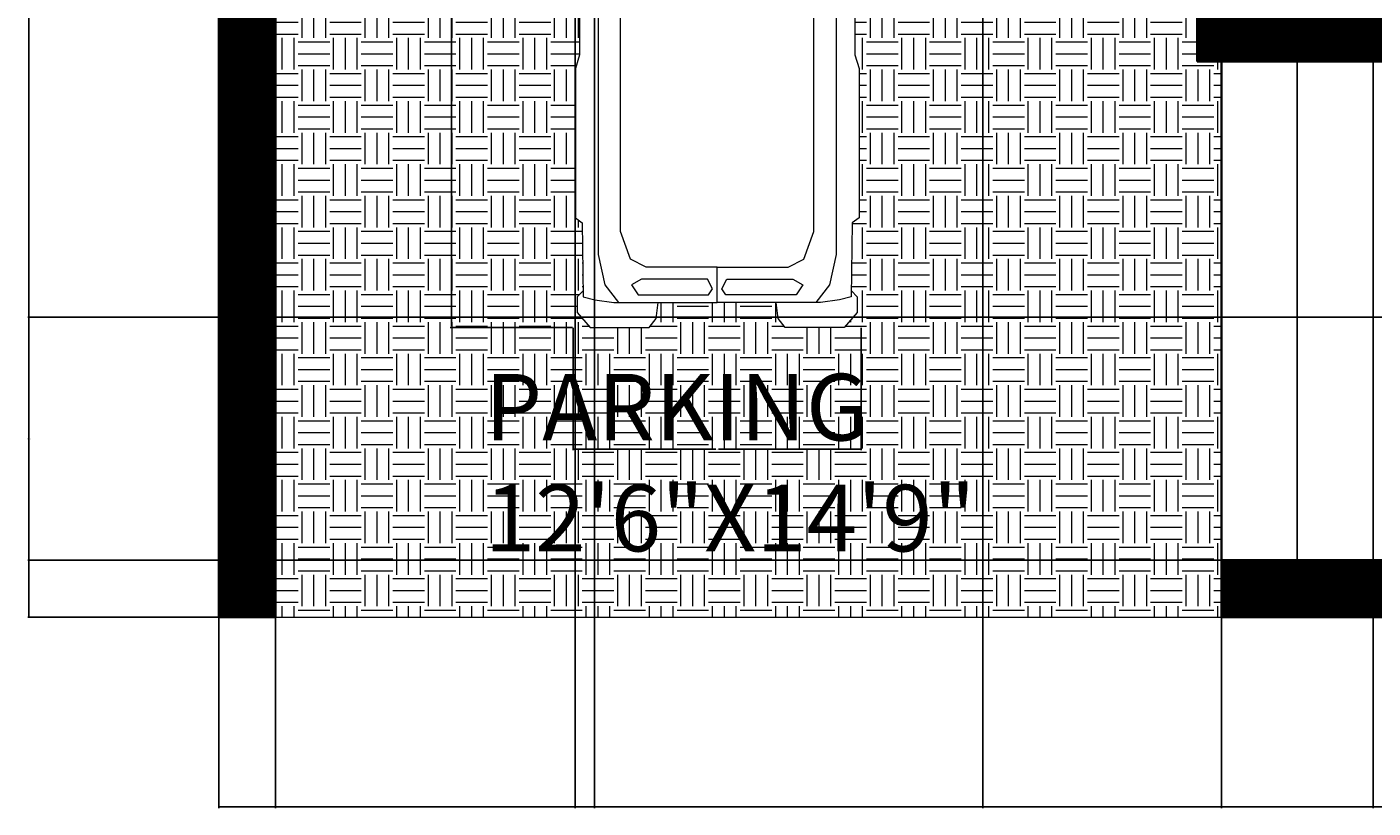
# Model space of a CAD drawing. Units: inches. Extents: x 205 to 1667, y -23 to 828.
# Tile 1 of 10: x 432 to 645, y -23 to 101. Entities that reach past the tile are written whole.
import ezdxf

# ---------------------------------------------------------------- set-up
doc = ezdxf.new("R2010")
doc.units = ezdxf.units.IN
doc.header["$MEASUREMENT"] = 0
for name, color, linetype, lineweight in [('A-ANNO-DIMS', 2, 'Continuous', 18), ('A-AREA-IDEN', 7, 'Continuous', 25), ('A-FLOR-PKNG', 8, 'Continuous', 18), ('A-FLOR-STRS', 7, 'Continuous', 25), ('A-WALL', 7, 'Continuous', 35)]:
    doc.layers.add(name, color=color, linetype=linetype, lineweight=lineweight)
doc.layers.add('A-FLOR-PATT', color=9, linetype='Continuous', lineweight=9, true_color=0xc7c8ca)
doc.styles.get("Standard").update_dxf_attribs({"font": 'arial.ttf'})
doc.dimstyles.get("Standard").update_dxf_attribs({"dimtxt": 0.18, "dimasz": 0.18, "dimexe": 0.18, "dimexo": 0.0625, "dimgap": 0.09, "dimtad": 0, "dimtih": 1, "dimtoh": 1, "dimdec": 4, "dimzin": 0, "dimdsep": 46, "dimtxsty": 'Standard', "dimcen": 0.09, "dimadec": 0, "dimazin": 0, "dimtfac": 1, "dimtdec": 4, "dimtofl": 0, "dimtmove": 0, "dimatfit": 3, "dimfxl": 1, "dimtolj": 1, "dimtzin": 0, "dimarcsym": 0})

# ---------------------------------------------------------------- blocks, each defined once
blk = doc.blocks.new('A$C3BDD66A0')
for p, q in [((-1.6934, 0.7345), (-1.7501, 0.6077)), ((-1.5608, 0.7448), (-1.6934, 0.7345)), ((-1.5055, 0.6573), (-1.5608, 0.7448)), ((-1.383, 0.6896), (-1.3262, 0.7247)), ((-1.3262, 0.7247), (-0.6328, 0.7247)), ((-0.6328, 0.7247), (-0.5818, 0.7108)), ((-0.5818, 0.7108), (1.0338, 0.7108)), ((0.0405, 0.522), (-0.2453, 0.7108)), ((1.0338, 0.7108), (1.1052, 0.7328)), ((1.1052, 0.7328), (1.8759, 0.7328)), ((1.8759, 0.7328), (1.9021, 0.6971)), ((1.9021, 0.6971), (2.2838, 0.6931)), ((2.2533, 0.6934), (2.2838, 0.7237)), ((2.2838, 0.7237), (2.3654, 0.7238)), ((2.3654, 0.7238), (2.4427, 0.6569)), ((-1.6379, 0.6224), (-1.383, 0.6896)), ((2.2838, 0.6931), (2.2999, 0.6319)), ((2.2999, 0.6319), (2.3146, 0.5344)), ((2.4427, 0.6569), (2.4427, 0.3509)), ((-1.7501, 0.6077), (-1.7501, 0)), ((-1.6275, 0.3471), (-1.6379, 0.6224)), ((-0.363, 0.4561), (-0.2962, 0.6237)), ((-0.363, 0.4561), (-0.2962, 0.6237)), ((-0.2962, 0.6237), (-0.2204, 0.599)), ((-0.2962, 0.6237), (-0.2204, 0.599)), ((-0.2204, 0.599), (0.0303, 0.4462)), ((-0.2204, 0.599), (0.0303, 0.4462)), ((-0.0842, 0.6044), (0.6056, 0.6044)), ((0.6056, 0.6044), (0.6056, 0.499)), ((0.6523, 0.6144), (2.0654, 0.6144)), ((0.6523, 0.499), (0.6523, 0.6144)), ((2.0654, 0.6144), (2.2228, 0.5809)), ((2.2228, 0.5809), (2.3146, 0.5096)), ((-1.6296, 0.403), (-1.0973, 0.5311)), ((-1.0973, 0.5311), (-0.4592, 0.5317)), ((-0.4592, 0.5317), (-0.4952, 0)), ((0.1935, 0.499), (0.0405, 0.522)), ((1.9475, 0.499), (0.1935, 0.499)), ((2.0903, 0.4482), (1.9475, 0.499)), ((2.3146, 0.5344), (2.3146, 0)), ((-0.4282, 0), (-0.363, 0.4561)), ((-0.4282, 0), (-0.363, 0.4561)), ((0.0303, 0.4462), (0.0654, 0.3691)), ((0.0303, 0.4462), (0.0654, 0.3691)), ((2.1315, 0.3666), (2.0903, 0.4482)), ((2.1927, 0.3914), (2.2229, 0.4425)), ((2.2229, 0.4425), (2.2739, 0.4076)), ((0.0654, 0.3691), (0, 0.1752)), ((0.0654, 0.3691), (0, 0.1752)), ((2.1315, 0), (2.1315, 0.3666)), ((2.1927, 0.0506), (2.1927, 0.3914)), ((2.2739, 0.4076), (2.2742, 0.0448)), ((2.4427, 0.3509), (2.3964, 0.3159)), ((-1.6519, 0), (-1.6275, 0.3471)), ((2.3964, 0.3159), (2.3146, 0.3056)), ((0, 0.1752), (0, 0)), ((0, 0.1752), (0, 0)), ((-1.7501, -0.6077), (-1.7501, 0)), ((-1.6519, 0), (-1.6275, -0.3471)), ((-1.4334, 0), (-0.4906, 0.0678)), ((-1.4334, 0), (-0.4906, -0.0678)), ((-0.4592, -0.5317), (-0.4952, 0)), ((-0.4282, 0), (-0.363, -0.4561)), ((-0.4282, 0), (-0.363, -0.4561)), ((0, -0.1752), (0, 0)), ((0, -0.1752), (0, 0)), ((2.1315, 0), (2.1315, -0.3666)), ((2.3146, 0), (2.1315, 0)), ((2.2437, 0.0244), (2.1927, 0.0506)), ((2.2742, 0.0448), (2.2437, 0.0244)), ((2.3146, -0.5344), (2.3146, 0)), ((2.2437, -0.0244), (2.1927, -0.0506)), ((2.1927, -0.0506), (2.1927, -0.3914)), ((2.2742, -0.0448), (2.2437, -0.0244)), ((2.2739, -0.4076), (2.2742, -0.0448)), ((0.0654, -0.3691), (0, -0.1752)), ((0.0654, -0.3691), (0, -0.1752)), ((-1.6275, -0.3471), (-1.6379, -0.6224)), ((2.3964, -0.3159), (2.3146, -0.3056)), ((2.4427, -0.3509), (2.3964, -0.3159)), ((-1.6296, -0.403), (-1.0973, -0.5311)), ((0.0303, -0.4462), (0.0654, -0.3691)), ((0.0303, -0.4462), (0.0654, -0.3691)), ((2.1315, -0.3666), (2.0903, -0.4482)), ((2.1927, -0.3914), (2.2229, -0.4425)), ((2.2229, -0.4425), (2.2739, -0.4076)), ((2.4427, -0.6569), (2.4427, -0.3509)), ((-0.363, -0.4561), (-0.2962, -0.6237)), ((-0.363, -0.4561), (-0.2962, -0.6237)), ((-0.2204, -0.599), (0.0303, -0.4462)), ((-0.2204, -0.599), (0.0303, -0.4462)), ((2.0903, -0.4482), (1.9475, -0.499)), ((-1.0973, -0.5311), (-0.4592, -0.5317)), ((0.0405, -0.522), (-0.2453, -0.7108)), ((0.1935, -0.499), (0.0405, -0.522)), ((1.9475, -0.499), (0.1935, -0.499)), ((0.6056, -0.6044), (0.6056, -0.499)), ((0.6523, -0.499), (0.6523, -0.6144)), ((2.2228, -0.5809), (2.3146, -0.5096)), ((2.2999, -0.6319), (2.3146, -0.5344)), ((-1.6934, -0.7345), (-1.7501, -0.6077)), ((-1.6379, -0.6224), (-1.383, -0.6896)), ((-0.2962, -0.6237), (-0.2204, -0.599)), ((-0.2962, -0.6237), (-0.2204, -0.599)), ((-0.0842, -0.6044), (0.6056, -0.6044)), ((0.6523, -0.6144), (2.0654, -0.6144)), ((2.0654, -0.6144), (2.2228, -0.5809)), ((-1.5055, -0.6573), (-1.5608, -0.7448)), ((-1.383, -0.6896), (-1.3262, -0.7247)), ((1.9021, -0.6971), (2.2838, -0.6931)), ((2.2533, -0.6934), (2.2838, -0.7237)), ((2.2838, -0.6931), (2.2999, -0.6319)), ((2.3654, -0.7238), (2.4427, -0.6569)), ((-1.5608, -0.7448), (-1.6934, -0.7345)), ((-1.3262, -0.7247), (-0.6328, -0.7247)), ((-0.6328, -0.7247), (-0.5818, -0.7108)), ((-0.5818, -0.7108), (1.0338, -0.7108)), ((1.0338, -0.7108), (1.1052, -0.7328)), ((1.1052, -0.7328), (1.8759, -0.7328)), ((1.8759, -0.7328), (1.9021, -0.6971)), ((2.2838, -0.7237), (2.3654, -0.7238))]:
    blk.add_line(p, q)
blk = doc.blocks.new('*D40')
at = {"layer": 'A-ANNO-DIMS', "color": 0, "lineweight": -2, "transparency": 16777216}
for p, q in [((518.48, 182.02), (499.09, 182.02)), ((499.27, 181.84), (499.27, 117.96)), ((499.27, 53.72), (499.27, 117.59)), ((518.48, 53.54), (499.09, 53.54))]:
    blk.add_line(p, q, dxfattribs=at)
at = {"layer": 'A-ANNO-DIMS', "color": 0, "transparency": 16777216}
for points in [[(499.24, 181.84), (499.3, 181.84), (499.27, 182.02)], [(499.24, 53.72), (499.3, 53.72), (499.27, 53.54)]]:
    blk.add_solid(points, dxfattribs=at)
at = {"layer": 'Defpoints', "color": 0, "transparency": 16777216}
for p in [(518.54, 182.02), (499.27, 53.54), (518.54, 53.54)]:
    blk.add_point(p, dxfattribs=at)
at = {"layer": 'A-ANNO-DIMS', "color": 0, "transparency": 16777216, "insert": (499.27, 117.78), "char_height": 0.18, "attachment_point": 5}
blk.add_mtext('\\A1;CAR 128', dxfattribs=at)
blk = doc.blocks.new('*D41')
at = {"layer": 'A-ANNO-DIMS', "color": 0, "lineweight": -2, "transparency": 16777216}
for p, q in [((518.54, 53.48), (518.54, 34.09)), ((564.19, 53.48), (564.19, 34.09)), ((518.72, 34.27), (541.14, 34.27)), ((564.01, 34.27), (541.59, 34.27))]:
    blk.add_line(p, q, dxfattribs=at)
at = {"layer": 'A-ANNO-DIMS', "color": 0, "transparency": 16777216}
for points in [[(518.72, 34.3), (518.72, 34.24), (518.54, 34.27)], [(564.01, 34.3), (564.01, 34.24), (564.19, 34.27)]]:
    blk.add_solid(points, dxfattribs=at)
at = {"layer": 'Defpoints', "color": 0, "transparency": 16777216}
for p in [(518.54, 53.54), (564.19, 53.54), (564.19, 34.27)]:
    blk.add_point(p, dxfattribs=at)
at = {"layer": 'A-ANNO-DIMS', "color": 0, "transparency": 16777216, "insert": (541.37, 34.27), "char_height": 0.18, "attachment_point": 5}
blk.add_mtext('\\A1;46', dxfattribs=at)
blk = doc.blocks.new('*D42')
at = {"layer": 'A-ANNO-DIMS', "color": 0, "lineweight": -2, "transparency": 16777216}
for p, q in [((462.43, 7.59), (462.43, -22.59)), ((774.43, 7.59), (774.43, -22.59)), ((462.61, -22.41), (618.14, -22.41)), ((774.25, -22.41), (618.72, -22.41))]:
    blk.add_line(p, q, dxfattribs=at)
at = {"layer": 'A-ANNO-DIMS', "color": 0, "transparency": 16777216}
for points in [[(462.61, -22.38), (462.61, -22.44), (462.43, -22.41)], [(774.25, -22.38), (774.25, -22.44), (774.43, -22.41)]]:
    blk.add_solid(points, dxfattribs=at)
at = {"layer": 'Defpoints', "color": 0, "transparency": 16777216}
for p in [(462.43, 7.65), (774.43, 7.65), (774.43, -22.41)]:
    blk.add_point(p, dxfattribs=at)
at = {"layer": 'A-ANNO-DIMS', "color": 0, "transparency": 16777216, "insert": (618.43, -22.41), "char_height": 0.18, "attachment_point": 5}
blk.add_mtext('\\A1;312', dxfattribs=at)
blk = doc.blocks.new('*D43')
at = {"layer": 'A-ANNO-DIMS', "color": 0, "lineweight": -2, "transparency": 16777216}
for p, q in [((462.37, 607.65), (432.19, 607.65)), ((432.37, 607.47), (432.37, 307.83)), ((432.37, 7.83), (432.37, 307.47)), ((462.37, 7.65), (432.19, 7.65))]:
    blk.add_line(p, q, dxfattribs=at)
at = {"layer": 'A-ANNO-DIMS', "color": 0, "transparency": 16777216}
for points in [[(432.34, 607.47), (432.4, 607.47), (432.37, 607.65)], [(432.34, 7.83), (432.4, 7.83), (432.37, 7.65)]]:
    blk.add_solid(points, dxfattribs=at)
at = {"layer": 'Defpoints', "color": 0, "transparency": 16777216}
for p in [(432.37, 607.65), (462.43, 607.65), (462.43, 7.65)]:
    blk.add_point(p, dxfattribs=at)
at = {"layer": 'A-ANNO-DIMS', "color": 0, "transparency": 16777216, "insert": (432.37, 307.65), "char_height": 0.18, "attachment_point": 5}
blk.add_mtext('\\A1;600', dxfattribs=at)
blk = doc.blocks.new('*D44')
at = {"layer": 'A-ANNO-DIMS', "color": 0, "lineweight": -2, "transparency": 16777216}
for p, q in [((462.43, 7.59), (462.43, -22.59)), ((621.22, 7.59), (621.22, -22.59)), ((462.61, -22.41), (541.44, -22.41)), ((621.04, -22.41), (542.21, -22.41))]:
    blk.add_line(p, q, dxfattribs=at)
at = {"layer": 'A-ANNO-DIMS', "color": 0, "transparency": 16777216}
for points in [[(462.61, -22.38), (462.61, -22.44), (462.43, -22.41)], [(621.04, -22.38), (621.04, -22.44), (621.22, -22.41)]]:
    blk.add_solid(points, dxfattribs=at)
at = {"layer": 'Defpoints', "color": 0, "transparency": 16777216}
for p in [(462.43, 7.65), (621.22, 7.65), (621.22, -22.41)]:
    blk.add_point(p, dxfattribs=at)
at = {"layer": 'A-ANNO-DIMS', "color": 0, "transparency": 16777216, "insert": (541.83, -22.41), "char_height": 0.18, "attachment_point": 5}
blk.add_mtext('\\A1;158.8', dxfattribs=at)
blk = doc.blocks.new('*D52')
at = {"layer": 'A-ANNO-DIMS', "color": 0, "lineweight": -2, "transparency": 16777216}
for p, q in [((471.43, 204.87), (471.43, -22.59)), ((521.94, 204.87), (521.94, -22.59)), ((471.61, -22.41), (496.36, -22.41)), ((521.76, -22.41), (497.01, -22.41))]:
    blk.add_line(p, q, dxfattribs=at)
at = {"layer": 'A-ANNO-DIMS', "color": 0, "transparency": 16777216}
for points in [[(471.61, -22.38), (471.61, -22.44), (471.43, -22.41)], [(521.76, -22.38), (521.76, -22.44), (521.94, -22.41)]]:
    blk.add_solid(points, dxfattribs=at)
at = {"layer": 'Defpoints', "color": 0, "transparency": 16777216}
for p in [(471.43, 204.93), (521.94, 204.93), (521.94, -22.41)]:
    blk.add_point(p, dxfattribs=at)
at = {"layer": 'A-ANNO-DIMS', "color": 0, "transparency": 16777216, "insert": (496.68, -22.41), "char_height": 0.18, "attachment_point": 5}
blk.add_mtext('\\A1;50.5', dxfattribs=at)
blk = doc.blocks.new('*D55')
at = {"layer": 'A-ANNO-DIMS', "color": 0, "lineweight": -2, "transparency": 16777216}
for p, q in [((621.22, 16.71), (621.22, 637.89)), ((621.4, 637.71), (627.01, 637.71)), ((633.04, 637.71), (627.43, 637.71)), ((633.22, 16.71), (633.22, 637.89))]:
    blk.add_line(p, q, dxfattribs=at)
at = {"layer": 'A-ANNO-DIMS', "color": 0, "transparency": 16777216}
for points in [[(621.4, 637.74), (621.4, 637.68), (621.22, 637.71)], [(633.04, 637.74), (633.04, 637.68), (633.22, 637.71)]]:
    blk.add_solid(points, dxfattribs=at)
at = {"layer": 'Defpoints', "color": 0, "transparency": 16777216}
for p in [(633.22, 637.71), (621.22, 16.65), (633.22, 16.65)]:
    blk.add_point(p, dxfattribs=at)
at = {"layer": 'A-ANNO-DIMS', "color": 0, "transparency": 16777216, "insert": (627.22, 637.71), "char_height": 0.18, "attachment_point": 5}
blk.add_mtext('\\A1;12', dxfattribs=at)
blk = doc.blocks.new('*D56')
at = {"layer": 'A-ANNO-DIMS', "color": 0, "lineweight": -2, "transparency": 16777216}
for p, q in [((621.16, 55.14), (432.19, 55.14)), ((432.37, 54.96), (432.37, 36.08)), ((432.37, 16.83), (432.37, 35.72)), ((621.16, 16.65), (432.19, 16.65))]:
    blk.add_line(p, q, dxfattribs=at)
at = {"layer": 'A-ANNO-DIMS', "color": 0, "transparency": 16777216}
for points in [[(432.34, 54.96), (432.4, 54.96), (432.37, 55.14)], [(432.34, 16.83), (432.4, 16.83), (432.37, 16.65)]]:
    blk.add_solid(points, dxfattribs=at)
at = {"layer": 'Defpoints', "color": 0, "transparency": 16777216}
for p in [(432.37, 55.14), (621.22, 55.14), (621.22, 16.65)]:
    blk.add_point(p, dxfattribs=at)
at = {"layer": 'A-ANNO-DIMS', "color": 0, "transparency": 16777216, "insert": (432.37, 35.9), "char_height": 0.18, "attachment_point": 5}
blk.add_mtext('\\A1;38.49', dxfattribs=at)
blk = doc.blocks.new('*D57')
at = {"layer": 'A-ANNO-DIMS', "color": 0, "lineweight": -2, "transparency": 16777216}
for p, q in [((621.22, 95.58), (621.22, -22.59)), ((645.22, 95.58), (645.22, -22.59)), ((621.4, -22.41), (633, -22.41)), ((645.04, -22.41), (633.44, -22.41))]:
    blk.add_line(p, q, dxfattribs=at)
at = {"layer": 'A-ANNO-DIMS', "color": 0, "transparency": 16777216}
for points in [[(621.4, -22.38), (621.4, -22.44), (621.22, -22.41)], [(645.04, -22.38), (645.04, -22.44), (645.22, -22.41)]]:
    blk.add_solid(points, dxfattribs=at)
at = {"layer": 'Defpoints', "color": 0, "transparency": 16777216}
for p in [(621.22, 95.64), (645.22, 95.64), (645.22, -22.41)]:
    blk.add_point(p, dxfattribs=at)
at = {"layer": 'A-ANNO-DIMS', "color": 0, "transparency": 16777216, "insert": (633.22, -22.41), "char_height": 0.18, "attachment_point": 5}
blk.add_mtext('\\A1;24', dxfattribs=at)
blk = doc.blocks.new('*D64')
at = {"layer": 'A-ANNO-DIMS', "color": 0, "lineweight": -2, "transparency": 16777216}
for p, q in [((471.43, 454.59), (471.43, -22.59)), ((583.44, 454.59), (583.44, -22.59)), ((471.61, -22.41), (527.16, -22.41)), ((583.26, -22.41), (527.71, -22.41))]:
    blk.add_line(p, q, dxfattribs=at)
at = {"layer": 'A-ANNO-DIMS', "color": 0, "transparency": 16777216}
for points in [[(471.61, -22.38), (471.61, -22.44), (471.43, -22.41)], [(583.26, -22.38), (583.26, -22.44), (583.44, -22.41)]]:
    blk.add_solid(points, dxfattribs=at)
at = {"layer": 'Defpoints', "color": 0, "transparency": 16777216}
for p in [(471.43, 454.65), (583.44, 454.65), (583.44, -22.41)]:
    blk.add_point(p, dxfattribs=at)
at = {"layer": 'A-ANNO-DIMS', "color": 0, "transparency": 16777216, "insert": (527.44, -22.41), "char_height": 0.18, "attachment_point": 5}
blk.add_mtext('\\A1;112', dxfattribs=at)
blk = doc.blocks.new('*D82')
at = {"layer": 'A-ANNO-DIMS', "color": 0, "lineweight": -2, "transparency": 16777216}
for p, q in [((471.43, 204.87), (471.43, -22.59)), ((518.86, 180.22), (518.86, -22.59)), ((471.61, -22.41), (494.75, -22.41)), ((518.68, -22.41), (495.54, -22.41))]:
    blk.add_line(p, q, dxfattribs=at)
at = {"layer": 'A-ANNO-DIMS', "color": 0, "transparency": 16777216}
for points in [[(471.61, -22.38), (471.61, -22.44), (471.43, -22.41)], [(518.68, -22.38), (518.68, -22.44), (518.86, -22.41)]]:
    blk.add_solid(points, dxfattribs=at)
at = {"layer": 'Defpoints', "color": 0, "transparency": 16777216}
for p in [(471.43, 204.93), (518.86, 180.28), (518.86, -22.41)]:
    blk.add_point(p, dxfattribs=at)
at = {"layer": 'A-ANNO-DIMS', "color": 0, "transparency": 16777216, "insert": (495.14, -22.41), "char_height": 0.18, "attachment_point": 5}
blk.add_mtext('\\A1;47.43', dxfattribs=at)
blk = doc.blocks.new('*D84')
at = {"layer": 'A-ANNO-DIMS', "color": 0, "lineweight": -2, "transparency": 16777216}
for p, q in [((471.37, 204.93), (432.19, 204.93)), ((432.37, 204.75), (432.37, 106.47)), ((432.37, 7.83), (432.37, 106.11)), ((471.37, 7.65), (432.19, 7.65))]:
    blk.add_line(p, q, dxfattribs=at)
at = {"layer": 'A-ANNO-DIMS', "color": 0, "transparency": 16777216}
for points in [[(432.34, 204.75), (432.4, 204.75), (432.37, 204.93)], [(432.34, 7.83), (432.4, 7.83), (432.37, 7.65)]]:
    blk.add_solid(points, dxfattribs=at)
at = {"layer": 'Defpoints', "color": 0, "transparency": 16777216}
for p in [(432.37, 204.93), (471.43, 204.93), (471.43, 7.65)]:
    blk.add_point(p, dxfattribs=at)
at = {"layer": 'A-ANNO-DIMS', "color": 0, "transparency": 16777216, "insert": (432.37, 106.29), "char_height": 0.18, "attachment_point": 5}
blk.add_mtext('\\A1;197.3', dxfattribs=at)

msp = doc.modelspace()

# ---------------------------------------------------------------- hatches: boundary and pattern name
at = {"layer": 'A-FLOR-PATT'}
h = msp.add_hatch(dxfattribs=at)
h.set_pattern_fill('ANSI31', color=256)
h.paths.add_polyline_path([(774.4305, 607.6511), (720.5338, 607.6511), (720.5338, 598.6511), (727.9933, 598.6511), (746.8614, 598.6511), (765.4305, 598.6511), (765.4305, 454.6511), (759.5298, 454.6511), (759.5298, 448.9635), (765.4305, 448.9635), (765.4305, 428.0602), (774.4305, 428.0602)])
h.paths.add_polyline_path([(765.4305, 598.6511), (746.8614, 598.6511), (746.8614, 579.7829), (727.9933, 579.7829), (727.9933, 518.1387, -0.41421701), (724.6389, 514.7843), (668.2693, 514.7843, -0.41421356), (665.0743, 517.9793), (665.0743, 579.7829), (646.2062, 579.7829), (646.2062, 598.6511), (626.3468, 598.6511), (626.3468, 454.6511), (628.3468, 454.6511), (628.3468, 484.9635, -0.41421356), (664.3468, 449.9635), (664.3468, 454.6511), (729.3305, 454.6511), (758.5298, 454.6511), (759.5298, 454.6511), (765.4305, 454.6511)])
h.paths.add_polyline_path([(621.4404, 598.6511), (471.4305, 598.6511), (471.4305, 568.8442), (490.2987, 568.8442), (490.2987, 549.9761), (551.9429, 549.9761, -0.41421701), (555.2973, 546.6217), (555.2973, 490.2521, -0.41421356), (552.1023, 487.0571), (490.2987, 487.0571), (490.2987, 468.189), (471.4305, 468.189), (471.4305, 454.6511), (583.4404, 454.6511), (583.4404, 449.9635, -0.41421356), (619.4404, 484.9635), (619.4404, 454.6511), (621.4404, 454.6511)])
h.paths.add_polyline_path([(672.5338, 607.6511), (569.5707, 607.6511), (569.5707, 598.6511), (621.4404, 598.6511), (621.4404, 454.6511), (619.4404, 454.6511), (619.4404, 448.9635), (628.3468, 448.9635), (628.3468, 454.6511), (626.3468, 454.6511), (626.3468, 598.6511), (646.2062, 598.6511), (665.0743, 598.6511), (672.5338, 598.6511)])
h.paths.add_polyline_path([(521.5707, 607.6511), (462.4305, 607.6511), (462.4305, 407.4306), (471.4305, 407.4306), (471.4305, 448.9635), (583.4404, 448.9635, -0.0070419), (583.4404, 449.9635), (583.4404, 454.6511), (471.4305, 454.6511), (471.4305, 468.189), (471.4305, 487.0571), (471.4305, 549.9761), (471.4305, 568.8442), (471.4305, 598.6511), (521.5707, 598.6511)])
h.paths.add_polyline_path([(471.4305, 314.3187), (583.4404, 314.3187), (583.4404, 319.9388), (471.4305, 319.9388), (471.4305, 359.4306), (462.4305, 359.4306), (462.4305, 7.6511), (471.4305, 7.6511), (471.4305, 204.9321), (521.9355, 204.9321), (521.9355, 213.9321), (471.4305, 213.9321)])
h.paths.add_polyline_path([(774.4305, 410.0602), (765.4305, 410.0602), (765.4305, 389.1569), (672.3024, 389.1569), (672.3024, 448.9635), (681.1739, 448.9635, -0.18532444), (681.6564, 449.1487), (698.6035, 449.1487), (729.3305, 448.9635), (729.3305, 454.6511), (664.3468, 454.6511), (664.3468, 449.9635, -0.0070419), (664.3468, 448.9635), (666.3024, 448.9635), (666.3024, 378.2485), (672.3024, 378.2485), (672.3024, 383.1306), (765.4305, 383.1306), (765.4305, 360.5347), (774.4305, 360.5347)])
h.paths.add_polyline_path([(774.4305, 342.5347), (765.4305, 342.5347), (765.4305, 319.9388), (672.3024, 319.9388), (672.3024, 348.5574), (671.0896, 348.5574, -0.04071533), (666.3024, 348.2485), (666.3024, 319.9388), (664.3468, 319.9388, -0.0070419), (664.3468, 318.9388), (664.3468, 314.3187), (765.4305, 314.3187), (765.4305, 290.8426), (774.4305, 290.8426)])
h.paths.add_polyline_path([(774.4305, 242.8426), (765.4305, 242.8426), (765.4305, 104.6382), (626.3468, 104.6382), (626.3468, 110.5917), (617.3468, 110.5917), (617.3468, 95.6382), (765.4305, 95.6382), (765.4305, 16.6511), (621.2232, 16.6511), (621.2232, 7.6511), (774.4305, 7.6511)])
h.paths.add_polyline_path([(626.3468, 314.3187), (628.3468, 314.3187), (628.3468, 319.9388), (619.4404, 319.9388), (619.4404, 314.3187), (620.4404, 314.3187), (620.4404, 213.9321), (569.9355, 213.9321), (569.9355, 204.9321), (617.3468, 204.9321), (617.3468, 153.3751), (626.3468, 153.3751)])
h.paths.add_polyline_path([(620.4404, 314.3187), (619.4404, 314.3187), (619.4404, 319.9388), (628.3468, 319.9388), (629.3468, 319.9388), (629.3468, 283.9388, 0.40598745), (664.3468, 318.9388), (664.3468, 319.9388), (666.3024, 319.9388), (666.3024, 348.2485), (666.3024, 377.2485), (666.3024, 378.2485), (666.3024, 448.9635), (664.3468, 448.9635), (664.3468, 449.9635, 0.40598745), (629.3468, 484.9635), (629.3468, 448.9635), (628.3468, 448.9635), (619.4404, 448.9635), (618.4404, 448.9635), (618.4404, 484.9635, 0.40598745), (583.4404, 449.9635), (583.4404, 448.9635), (471.4305, 448.9635), (471.4305, 407.4306), (471.4305, 359.4306), (471.4305, 319.9388), (583.4404, 319.9388), (583.4404, 314.3187), (495.4305, 314.3187), (495.4305, 237.9321), (620.4404, 237.9321)])
h.paths.add_polyline_path([(525.0876, 347.7863), (513.5657, 347.7863), (512.0216, 362.1672), (526.6317, 362.1672)], flags=16)
h.paths.add_polyline_path([(550.9499, 370.1471), (536.569, 368.6029), (536.569, 383.2131), (550.9499, 381.6689)], flags=16)
h.paths.add_polyline_path([(530.7713, 364.5431), (508.0415, 364.5431, -0.41421356), (504.7944, 367.7902), (504.7944, 403.5085, -0.41421356), (508.0415, 406.7556), (530.7713, 406.7556, -0.41421356), (534.0184, 403.5085), (534.0184, 367.7902, -0.41421356)], flags=16)
h.paths.add_polyline_path([(550.9499, 389.6298), (536.569, 388.0856), (536.569, 402.6958), (550.9499, 401.1516)], flags=16)
h.paths.add_polyline_path([(502.2439, 368.6029), (487.863, 370.1471), (487.863, 381.6689), (502.2439, 383.2131)], flags=16)
h.paths.add_polyline_path([(502.2439, 388.0856), (487.863, 389.6298), (487.863, 401.1516), (502.2439, 402.6958)], flags=16)
h.paths.add_polyline_path([(526.6317, 409.1315), (512.0216, 409.1315), (513.5657, 423.5124), (525.0876, 423.5124)], flags=16)
h.paths.add_polyline_path([(765.4305, 290.8426), (765.4305, 314.3187), (664.3468, 314.3187), (664.3468, 318.9388, -0.41421356), (628.3468, 283.9388), (628.3468, 314.3187), (626.3468, 314.3187), (626.3468, 153.3751), (638.3468, 153.3751, -0.4196361), (617.5748, 131.9834, -0.4196361), (638.3468, 110.5917), (626.3468, 110.5917), (626.3468, 104.6382), (765.4305, 104.6382), (765.4305, 242.8426)])
h.paths.add_polyline_path([(691.5064, 243.4363), (693.2483, 243.4363), (725.4984, 243.4363), (725.4984, 241.7329), (725.4984, 177.0512), (723.7564, 177.0512), (691.5064, 177.0512), (691.5064, 178.7545)], flags=16)
h.paths.add_polyline_path([(689.8658, 265.2977), (689.8658, 296.6873, -0.41421356), (690.8346, 297.6561), (724.6111, 297.6561, -0.41421356), (725.5799, 296.6873), (725.5799, 265.2977, -0.41421356), (724.6111, 264.3289), (690.8346, 264.3289, -0.41421356)], flags=16)
h.paths.add_polyline_path([(694.1286, 265.6852), (694.1286, 288.9368, -0.41421356), (695.0974, 289.9056), (720.3483, 289.9056, -0.41421356), (721.3171, 288.9368), (721.3171, 265.6852, -0.04533947), (721.3013, 265.5106, -0.3531705), (720.3282, 264.7164), (695.0974, 264.7164, -0.41421356)], flags=0)
h.paths.add_polyline_path([(694.1286, 291.2619), (694.1286, 294.7497, -0.41421356), (695.0974, 295.7185), (720.3483, 295.7185, -0.41421356), (721.3171, 294.7497), (721.3171, 291.2619, -0.41421356), (720.3483, 290.2931), (695.0974, 290.2931, -0.41421356)], flags=0)
h.paths.add_polyline_path([(734.4369, 244.6615, -0.41421356), (735.2682, 245.4928), (762.2019, 245.4928, -0.41421356), (763.0332, 244.6615), (763.0332, 168.183, -0.41421356), (762.2019, 167.3517), (735.2682, 167.3517, -0.41421356), (734.4369, 168.183)], flags=16)
h.paths.add_polyline_path([(761.7032, 242.1676), (761.7032, 170.6768), (735.6007, 171.0093, -0.41421356), (734.7694, 171.8406), (734.7694, 193.5102, -0.56972741), (735.6007, 194.674, -0.41421356), (734.7694, 195.5053), (734.7694, 217.3423, -0.56972741), (735.6007, 218.5061, -0.41421356), (734.7694, 219.3374), (734.7694, 241.0038, -0.41421356), (735.6007, 241.8351), (735.1643, 242.1676)], flags=16)
h.paths.add_polyline_path([(757.5467, 171.0093), (760.5393, 171.0093, 0.41421356), (761.3706, 171.8406), (761.3706, 193.5102, 0.41421356), (760.5393, 194.3415), (757.5467, 194.3415, 0.41421356), (756.7154, 193.5102), (756.7155, 171.8534, 0.41871477)], flags=0)
h.paths.add_polyline_path([(756.7154, 241.0038, -0.41421356), (757.5467, 241.8351), (760.5393, 241.8351, -0.41421356), (761.3706, 241.0038), (761.3706, 219.3374, -0.41421356), (760.5393, 218.5061), (760.5393, 218.1736, -0.41421356), (761.3706, 217.3423), (761.3706, 195.5053, -0.41421356), (760.5393, 194.674), (757.5467, 194.674, -0.56972741), (756.3829, 195.5053, -0.41421356), (755.5516, 194.674), (755.5516, 194.3415, -0.41421356), (756.3829, 193.5102), (756.7154, 171.8406), (756.3829, 193.5102, 0.41421356), (755.5516, 194.3415), (735.6007, 194.674), (755.5516, 194.674, 0.41421356), (756.3829, 195.5053), (756.3829, 217.3423, 0.41421356), (755.5516, 218.1736), (735.6007, 218.5061), (755.5516, 218.5061, 0.41421356), (756.3829, 219.3374)], flags=0)
h.paths.add_polyline_path([(694.5151, 150.3608), (728.2916, 150.3608, -0.41421356), (729.2604, 149.3919), (729.2604, 118.0023, -0.41421356), (728.2916, 117.0335), (694.5151, 117.0335, -0.41421356), (693.5463, 118.0023), (693.5463, 149.3919, -0.41421356)], flags=16)
h.paths.add_polyline_path([(724.0288, 149.9732, -0.41421356), (724.9977, 149.0044), (724.9977, 125.7529, -0.41421356), (724.0288, 124.784), (698.7779, 124.784, -0.41421356), (697.8091, 125.7529), (697.8091, 149.0044, -0.04533947), (697.825, 149.179, -0.3531705), (698.798, 149.9732)], flags=0)
h.paths.add_polyline_path([(698.7779, 124.3965), (724.0288, 124.3965, -0.41421356), (724.9977, 123.4277), (724.9977, 119.94, -0.41421356), (724.0288, 118.9711), (698.7779, 118.9711, -0.41421356), (697.8091, 119.94), (697.8091, 123.4277, -0.41421356)], flags=0)
h = msp.add_hatch(dxfattribs=at)
h.set_pattern_fill('EARTH', color=256, scale=20)
h.paths.add_polyline_path([(617.3468, 204.9321), (471.4305, 204.9321), (471.4305, 7.6511), (621.2232, 7.6511), (621.2232, 95.6382), (617.3468, 95.6382), (617.3468, 110.5917), (617.3468, 111.5917)])
h.paths.add_polyline_path([(564.1913, 176.2169), (561.5098, 174.5217), (562.5, 170.769), (563.5731, 169.029), (563.5731, 147.7805), (563.1483, 146.2164), (563.1483, 96.7087), (563.8223, 94.5214), (563.8223, 70.9058), (562.7294, 70.1011), (562.6164, 59.3401), (563.5441, 58.4056), (563.5465, 55.9057), (561.4952, 53.5377), (552.1213, 53.5377), (551.0475, 54.9563), (550.7331, 57.4626), (541.3672, 57.4626), (532.0012, 57.4626), (531.6868, 54.9563), (530.613, 53.5377), (521.2392, 53.5377), (519.1879, 55.9057), (519.1903, 58.4056), (520.1179, 59.3401), (520.0049, 70.1011), (518.912, 70.9058), (518.912, 94.5214), (519.5861, 96.7087), (519.5861, 146.2164), (519.1613, 147.7805), (519.1613, 169.029), (520.2343, 170.769), (521.2245, 174.5217), (518.5431, 176.2169), (518.8594, 180.2791), (522.745, 182.0164), (541.3672, 182.0164), (559.9894, 182.0164), (563.8749, 180.2791)], flags=16)
h.paths.add_polyline_path([(553.7175, 178.3241), (557.6423, 162.0145), (557.6609, 142.4613), (541.3672, 143.5621), (525.0735, 142.4613), (525.092, 162.0145), (529.0169, 178.3241), (530.7323, 178.2589), (541.3672, 179.0078), (552.002, 178.2589)], flags=0)
h.paths.add_polyline_path([(560.4781, 137.464), (559.7214, 135.1419), (555.0412, 127.459), (552.6762, 126.3854), (546.7369, 128.3886), (541.3672, 128.3886), (535.9975, 128.3886), (530.0582, 126.3854), (527.6931, 127.459), (523.013, 135.1419), (522.2563, 137.464), (527.3921, 139.5127), (541.3672, 141.5088), (555.3423, 139.5127)], flags=0)
h.paths.add_polyline_path([(559.8869, 130.9684), (559.8869, 109.832), (556.6594, 109.832), (556.6594, 68.7114), (555.1011, 64.335), (552.6025, 63.0718), (541.3672, 63.0718), (530.1319, 63.0718), (527.6333, 64.335), (526.075, 68.7114), (526.075, 109.832), (522.8474, 109.832), (522.8474, 130.9684), (525.3715, 127.1487), (526.075, 122.4588), (526.075, 68.7114), (527.6333, 64.335), (530.1319, 63.0718), (541.3672, 63.0718), (552.6025, 63.0718), (555.1011, 64.335), (556.6594, 68.7114), (556.6594, 122.4588), (557.3629, 127.1487)], flags=0)
h.paths.add_polyline_path([(553.3621, 61.1985), (554.9264, 60.2724), (553.8564, 58.7089), (542.7405, 58.6984), (542.1147, 59.6353), (542.9167, 61.1985)], flags=0)
h.paths.add_polyline_path([(539.8176, 61.1985), (540.6197, 59.6353), (539.9938, 58.6984), (528.8779, 58.7089), (527.808, 60.2724), (529.3722, 61.1985)], flags=0)

# ---------------------------------------------------------------- linework, layer by layer
at = {"layer": 'A-FLOR-PKNG'}
msp.add_line((471.4305, 7.6511), (621.2232, 7.6511), dxfattribs=at)
at = {"layer": 'A-FLOR-STRS'}
for p, q in [((729.2232, 55.1446), (621.2232, 55.1446)), ((633.2232, 16.6511), (633.2232, 55.1446))]:
    msp.add_line(p, q, dxfattribs=at)
at = {"layer": 'A-WALL'}
for p, q in [((462.4305, 607.6511), (462.4305, 7.6511)), ((471.4305, 204.9321), (471.4305, 7.6511)), ((617.3468, 110.5917), (617.3468, 95.6382)), ((765.4305, 95.6382), (617.3468, 95.6382)), ((621.2232, 7.6511), (621.2232, 95.6382)), ((621.2232, 16.6511), (765.4305, 16.6511)), ((462.4305, 7.6511), (471.4305, 7.6511)), ((621.2232, 7.6511), (774.4305, 7.6511))]:
    msp.add_line(p, q, dxfattribs=at)

# ---------------------------------------------------------------- block references
at = {"layer": 'A-FLOR-PKNG', "xscale": 30.6431746435358, "yscale": 30.6431746435358, "zscale": 30.6431746435358, "rotation": 270}
msp.add_blockref('A$C3BDD66A0', (541.3672, 128.3886), dxfattribs=at)

# ---------------------------------------------------------------- texts
at = {"layer": 'A-AREA-IDEN', "insert": (504.551, 46.1776), "char_height": 10.539409, "attachment_point": 1}
msp.add_mtext_dynamic_manual_height_columns('PARKING\\P12\'6"X14\'9"', width=126.149246, gutter_width=52.697, heights=[33.1491], dxfattribs=at)

# ---------------------------------------------------------------- dimensions: what is measured, and where the dimension line sits
at = {"layer": 'A-ANNO-DIMS'}
for base, p1, p2, override, picture, middle in [((633.2232, 637.7086), (621.2232, 16.6511), (633.2232, 16.6511), {"dimdec": 0, "dimlfac": 1, "dimrnd": 0, "dimzin": 0, "dimdsep": 46, "dimlunit": 2}, '*D55', (627.2232, 637.7086)), ((583.4404, -22.4064), (471.4305, 454.6511), (583.4404, 454.6511), {"dimdec": 0, "dimlfac": 1, "dimrnd": 0, "dimzin": 0, "dimdsep": 46, "dimlunit": 2}, '*D64', (527.4355, -22.4064)), ((521.9355, -22.4064), (471.4305, 204.9321), (521.9355, 204.9321), {"dimdec": 1, "dimlfac": 1, "dimrnd": 0, "dimzin": 0, "dimdsep": 46, "dimlunit": 2}, '*D52', (496.683, -22.4064)), ((518.8594, -22.4064), (471.4305, 204.9321), (518.8594, 180.2791), {"dimdec": 2, "dimlfac": 1, "dimrnd": 0, "dimzin": 0, "dimdsep": 46, "dimlunit": 2}, '*D82', (495.145, -22.4064)), ((645.2232, -22.4064), (621.2232, 95.6382), (645.2232, 95.6382), {"dimdec": 0, "dimlfac": 1, "dimrnd": 0, "dimzin": 0, "dimdsep": 46, "dimlunit": 2}, '*D57', (633.2232, -22.4064)), ((564.1913, 34.2659), (518.5431, 53.5377), (564.1913, 53.5377), {"dimdec": 0, "dimlfac": 1, "dimrnd": 0, "dimzin": 0, "dimdsep": 46, "dimlunit": 2}, '*D41', (541.3672, 34.2659)), ((774.4305, -22.4064), (462.4305, 7.6511), (774.4305, 7.6511), {"dimdec": 0, "dimlfac": 1, "dimrnd": 0, "dimzin": 0, "dimdsep": 46, "dimlunit": 2}, '*D42', (618.4306, -22.4064)), ((621.2232, -22.4064), (462.4305, 7.6511), (621.2232, 7.6511), {"dimdec": 1, "dimlfac": 1, "dimrnd": 0, "dimzin": 0, "dimdsep": 46, "dimlunit": 2}, '*D44', (541.8269, -22.4064))]:
    dim = msp.add_linear_dim(base=base, p1=p1, p2=p2, dimstyle='Standard', override=override, dxfattribs=at)
    dim.commit()
    dim.dimension.update_dxf_attribs({"geometry": picture, "text_midpoint": middle})
for base, p1, p2, override, picture, middle in [((432.3731, 607.6511), (462.4305, 7.6511), (462.4305, 607.6511), {"dimdec": 0, "dimlfac": 1, "dimrnd": 0, "dimzin": 0, "dimdsep": 46, "dimlunit": 2}, '*D43', (432.3731, 307.6511)), ((432.3731, 204.9321), (471.4305, 7.6511), (471.4305, 204.9321), {"dimdec": 1, "dimlfac": 1, "dimrnd": 0, "dimzin": 0, "dimdsep": 46, "dimlunit": 2}, '*D84', (432.3731, 106.2916)), ((432.3731, 55.1446), (621.2232, 16.6511), (621.2232, 55.1446), {"dimdec": 2, "dimlfac": 1, "dimrnd": 0, "dimzin": 0, "dimdsep": 46, "dimlunit": 2}, '*D56', (432.3731, 35.8979))]:
    dim = msp.add_linear_dim(base=base, p1=p1, p2=p2, angle=90, dimstyle='Standard', override=override, dxfattribs=at)
    dim.commit()
    dim.dimension.update_dxf_attribs({"geometry": picture, "text_midpoint": middle})
dim = msp.add_linear_dim(base=(499.2713, 53.5377), p1=(518.5431, 182.0164), p2=(518.5431, 53.5377), angle=270, text='CAR <>', dimstyle='Standard', override={"dimdec": 0, "dimlfac": 1, "dimrnd": 0, "dimzin": 0, "dimdsep": 46, "dimlunit": 2}, dxfattribs=at)
dim.commit()
dim.dimension.update_dxf_attribs({"geometry": '*D40', "text_midpoint": (499.2713, 117.7771)})

doc.saveas('drawing.dxf')
